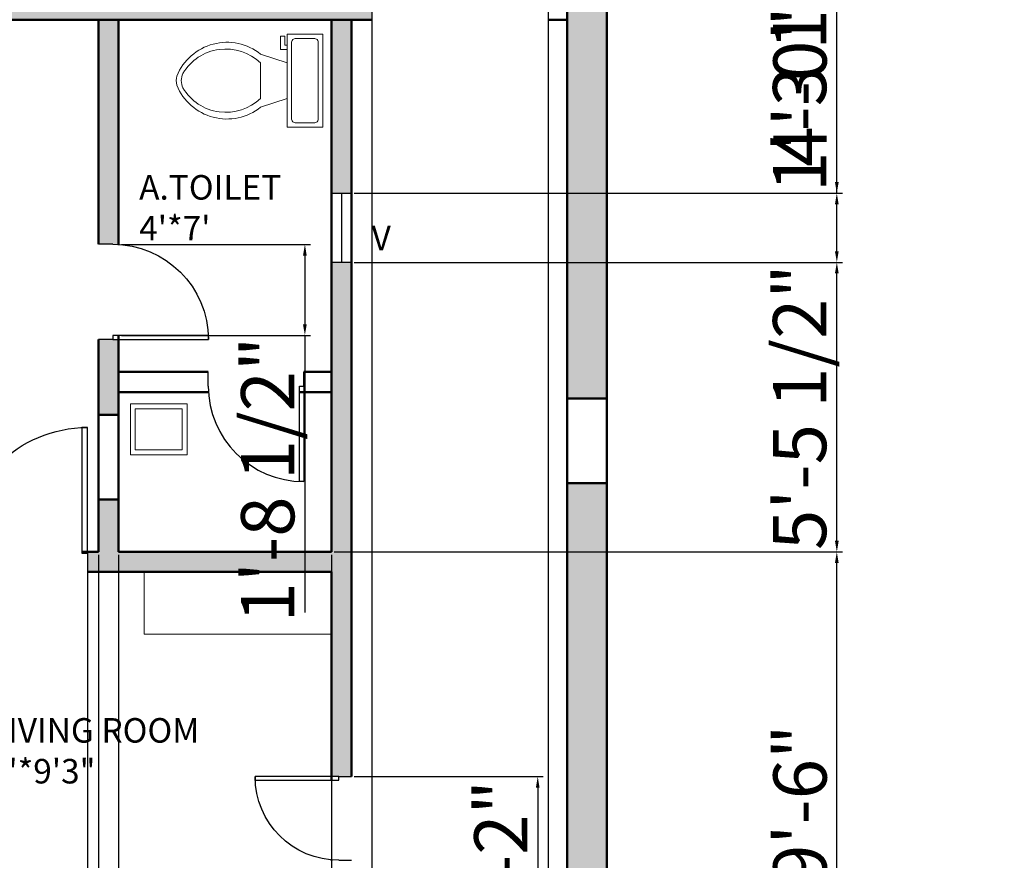
# Model space of a CAD drawing. Units: inches. Extents: x 2063 to 3370, y 2091 to 2971.
# Tile 5 of 14: x 2710 to 2932, y 2279 to 2468. Entities that reach past the tile are written whole.
import ezdxf

# ---------------------------------------------------------------- set-up
doc = ezdxf.new("R2010")
doc.units = ezdxf.units.IN
for name, color, linetype, lineweight in [('A-ANNO-DIMS', 2, 'Continuous', 18), ('A-ANNO-TEXT', 7, 'Continuous', 18), ('A-AREA-IDEN', 3, 'Continuous', 18), ('A-COLS', 7, 'Continuous', 50), ('A-DOOR', 4, 'Continuous', 25), ('A-FLOR-FIXT', 9, 'Continuous', 18), ('A-FURN', 8, 'Continuous', 18), ('A-GLAZ', 131, 'Continuous', 25), ('A-WALL', 7, 'Continuous', 50), ('A-WALL-PATT', 8, 'Continuous', 13)]:
    doc.layers.add(name, color=color, linetype=linetype, lineweight=lineweight)
doc.styles.get("Standard").update_dxf_attribs({"font": 'arial.ttf'})
doc.dimstyles.new('ISO-25', dxfattribs={"dimtxt": 12, "dimasz": 2.5, "dimexe": 1.25, "dimexo": 0.625, "dimtad": 1, "dimdec": 0, "dimlunit": 4, "dimtxsty": 'Standard', "dimcen": 2.5, "dimadec": 0, "dimazin": 0, "dimtfac": 1, "dimtdec": 0, "dimtmove": 0, "dimatfit": 3, "dimfxl": 1, "dimarcsym": 0})

# ---------------------------------------------------------------- blocks, each defined once
blk = doc.blocks.new('*U2')
for p, q in [((0, 0), (0, -6)), ((40, 0), (40, -6))]:
    blk.add_line(p, q)
blk.add_lwpolyline([(0, 0), (0, 40), (1.75, 40), (1.75, 0)], close=True)
blk.add_arc((0, 0), 40, 0, 90)
blk = doc.blocks.new('*U4')
for p, q in [((9.5, -6), (9.5, -2)), ((-10, -8.5), (-8, -8.5)), ((-10, -9.5), (-10, -8.5)), ((-8, -8.5), (-8, -8)), ((-7, -8), (-7, -9.5)), ((-4, -8), (-6, -14)), ((4, -8), (6, -14)), ((-7, -9.5), (-10, -9.5)), ((4, -14), (-4, -14))]:
    blk.add_line(p, q)
blk.add_lwpolyline([(10.5, -8), (10.5, 0), (-10.5, 0), (-10.5, -8)], close=True)
for points in [[(-9.5, -2), (-9.5, -6)], [(8.5, -1), (-8.5, -1)], [(-8.5, -7), (8.5, -7)]]:
    blk.add_lwpolyline(points)
for centre, radius, start, end in [((-8.62, -1.88), 0.884, 81.8699, 188.1301), ((8.62, -1.88), 0.884, 351.8699, 98.1301), ((-8.62, -6.12), 0.884, 171.8699, 278.1301), ((8.62, -6.12), 0.884, 261.8699, 8.1301), ((3.52, -21.58), 12.17, 141.4691, 247.9714), ((4.2, -21.82), 11.33, 136.3677, 238.9468), ((-3.52, -21.58), 12.17, 292.0284, 38.5307), ((-4.2, -21.82), 11.33, 301.053, 43.6321), ((0, -27.88), 4, 245.7318, 294.2682), ((0, -29), 4, 254.8605, 285.1395)]:
    blk.add_arc(centre, radius, start, end)
blk = doc.blocks.new('*D18')
at = {"layer": 'A-ANNO-DIMS', "color": 0, "lineweight": -2, "transparency": 16777216}
for p, q in [((2717.43, 2255.3), (2717.43, 2259.55)), ((2719.93, 2258.3), (2739.08, 2258.3)), ((2741.58, 2255.3), (2741.58, 2259.55)), ((2741.58, 2258.3), (2932.33, 2258.3))]:
    blk.add_line(p, q, dxfattribs=at)
at = {"layer": 'A-ANNO-DIMS', "color": 0, "transparency": 16777216}
for points in [[(2719.93, 2258.72), (2719.93, 2257.88), (2717.43, 2258.3)], [(2739.08, 2258.72), (2739.08, 2257.88), (2741.58, 2258.3)]]:
    blk.add_solid(points, dxfattribs=at)
at = {"layer": 'Defpoints', "color": 0, "transparency": 16777216}
for p in [(2741.58, 2258.3), (2717.43, 2254.68), (2741.58, 2254.68)]:
    blk.add_point(p, dxfattribs=at)
at = {"layer": 'A-ANNO-DIMS', "color": 0, "transparency": 16777216, "insert": (2838.21, 2265.13), "char_height": 12, "attachment_point": 5}
blk.add_mtext('2-SEAT SOFA 2\'-0" TYP.', dxfattribs=at)
blk = doc.blocks.new('*D28')
at = {"layer": 'A-ANNO-DIMS', "color": 0, "lineweight": -2, "transparency": 16777216}
for p, q in [((2647.53, 2480.55), (2647.53, 2476.06)), ((2673.28, 2480.55), (2673.28, 2476.06)), ((2650.03, 2477.31), (2670.78, 2477.31)), ((2673.28, 2477.31), (2793.91, 2477.31))]:
    blk.add_line(p, q, dxfattribs=at)
at = {"layer": 'A-ANNO-DIMS', "color": 0, "transparency": 16777216}
for points in [[(2650.03, 2477.73), (2650.03, 2476.9), (2647.53, 2477.31)], [(2670.78, 2477.73), (2670.78, 2476.9), (2673.28, 2477.31)]]:
    blk.add_solid(points, dxfattribs=at)
at = {"layer": 'Defpoints', "color": 0, "transparency": 16777216}
for p in [(2647.53, 2481.18), (2673.28, 2481.18), (2673.28, 2477.31)]:
    blk.add_point(p, dxfattribs=at)
at = {"layer": 'A-ANNO-DIMS', "color": 0, "transparency": 16777216, "insert": (2734.85, 2484.14), "char_height": 12, "attachment_point": 5}
blk.add_mtext('SINK 2\'-2" TYP.', dxfattribs=at)
blk = doc.blocks.new('*D94')
at = {"layer": 'A-ANNO-DIMS', "color": 0, "lineweight": -2, "transparency": 16777216}
for p, q in [((2611.75, 2347.8), (2611.75, 2101.18)), ((2728.14, 2347.8), (2728.14, 2101.18)), ((2614.25, 2102.43), (2725.64, 2102.43))]:
    blk.add_line(p, q, dxfattribs=at)
at = {"layer": 'A-ANNO-DIMS', "color": 0, "transparency": 16777216}
for points in [[(2614.25, 2102.84), (2614.25, 2102.01), (2611.75, 2102.43)], [(2725.64, 2102.84), (2725.64, 2102.01), (2728.14, 2102.43)]]:
    blk.add_solid(points, dxfattribs=at)
at = {"layer": 'Defpoints', "color": 0, "transparency": 16777216}
for p in [(2611.75, 2348.43), (2728.14, 2348.43), (2728.14, 2102.43)]:
    blk.add_point(p, dxfattribs=at)
at = {"layer": 'A-ANNO-DIMS', "color": 0, "transparency": 16777216, "insert": (2669.94, 2109.26), "char_height": 12, "attachment_point": 5}
blk.add_mtext('9\'-8 1/2"', dxfattribs=at)
blk = doc.blocks.new('*D95')
at = {"layer": 'A-ANNO-DIMS', "color": 0, "lineweight": -2, "transparency": 16777216}
for p, q in [((2728.14, 2347.8), (2728.14, 2101.18)), ((2732.64, 2347.8), (2732.64, 2101.18)), ((2725.64, 2102.43), (2723.14, 2102.43)), ((2728.14, 2102.43), (2732.64, 2102.43)), ((2735.14, 2102.43), (2798.75, 2102.43))]:
    blk.add_line(p, q, dxfattribs=at)
at = {"layer": 'A-ANNO-DIMS', "color": 0, "transparency": 16777216}
for points in [[(2725.64, 2102.84), (2725.64, 2102.01), (2728.14, 2102.43)], [(2735.14, 2102.84), (2735.14, 2102.01), (2732.64, 2102.43)]]:
    blk.add_solid(points, dxfattribs=at)
at = {"layer": 'Defpoints', "color": 0, "transparency": 16777216}
for p in [(2728.14, 2348.43), (2732.64, 2348.43), (2732.64, 2102.43)]:
    blk.add_point(p, dxfattribs=at)
at = {"layer": 'A-ANNO-DIMS', "color": 0, "transparency": 16777216, "insert": (2768.19, 2109.26), "char_height": 12, "attachment_point": 5}
blk.add_mtext('0\'-4 1/2"', dxfattribs=at)
blk = doc.blocks.new('*D96')
at = {"layer": 'A-ANNO-DIMS', "color": 0, "lineweight": -2, "transparency": 16777216}
for p, q in [((2732.64, 2347.8), (2732.64, 2101.18)), ((2780.64, 2347.8), (2780.64, 2101.18)), ((2735.14, 2102.43), (2778.14, 2102.43))]:
    blk.add_line(p, q, dxfattribs=at)
at = {"layer": 'A-ANNO-DIMS', "color": 0, "transparency": 16777216}
for points in [[(2735.14, 2102.84), (2735.14, 2102.01), (2732.64, 2102.43)], [(2778.14, 2102.84), (2778.14, 2102.01), (2780.64, 2102.43)]]:
    blk.add_solid(points, dxfattribs=at)
at = {"layer": 'Defpoints', "color": 0, "transparency": 16777216}
for p in [(2732.64, 2348.43), (2780.64, 2348.43), (2780.64, 2102.43)]:
    blk.add_point(p, dxfattribs=at)
at = {"layer": 'A-ANNO-DIMS', "color": 0, "transparency": 16777216, "insert": (2756.64, 2109.18), "char_height": 12, "attachment_point": 5}
blk.add_mtext('4\'-0"', dxfattribs=at)
blk = doc.blocks.new('*D113')
at = {"layer": 'A-ANNO-DIMS', "color": 0, "lineweight": -2, "transparency": 16777216}
for p, q in [((2781.26, 2348.43), (2895.82, 2348.43)), ((2894.57, 2236.93), (2894.57, 2345.93)), ((2781.26, 2234.43), (2895.82, 2234.43))]:
    blk.add_line(p, q, dxfattribs=at)
at = {"layer": 'A-ANNO-DIMS', "color": 0, "transparency": 16777216}
for points in [[(2894.15, 2345.93), (2894.99, 2345.93), (2894.57, 2348.43)], [(2894.15, 2236.93), (2894.99, 2236.93), (2894.57, 2234.43)]]:
    blk.add_solid(points, dxfattribs=at)
at = {"layer": 'Defpoints', "color": 0, "transparency": 16777216}
for p in [(2780.64, 2348.43), (2894.57, 2348.43), (2780.64, 2234.43)]:
    blk.add_point(p, dxfattribs=at)
at = {"layer": 'A-ANNO-DIMS', "color": 0, "transparency": 16777216, "insert": (2887.82, 2291.43), "char_height": 12, "attachment_point": 5, "rotation": 90}
blk.add_mtext('9\'-6"', dxfattribs=at)
blk = doc.blocks.new('*D114')
at = {"layer": 'A-ANNO-DIMS', "color": 0, "lineweight": -2, "transparency": 16777216}
for p, q in [((2785.76, 2413.72), (2895.82, 2413.72)), ((2894.57, 2350.93), (2894.57, 2411.22)), ((2781.26, 2348.43), (2895.82, 2348.43))]:
    blk.add_line(p, q, dxfattribs=at)
at = {"layer": 'A-ANNO-DIMS', "color": 0, "transparency": 16777216}
for points in [[(2894.15, 2411.22), (2894.99, 2411.22), (2894.57, 2413.72)], [(2894.15, 2350.93), (2894.99, 2350.93), (2894.57, 2348.43)]]:
    blk.add_solid(points, dxfattribs=at)
at = {"layer": 'Defpoints', "color": 0, "transparency": 16777216}
for p in [(2785.14, 2413.72), (2894.57, 2413.72), (2780.64, 2348.43)]:
    blk.add_point(p, dxfattribs=at)
at = {"layer": 'A-ANNO-DIMS', "color": 0, "transparency": 16777216, "insert": (2887.74, 2381.07), "char_height": 12, "attachment_point": 5, "rotation": 90}
blk.add_mtext('5\'-5 1/2"', dxfattribs=at)
blk = doc.blocks.new('*D115')
at = {"layer": 'A-ANNO-DIMS', "color": 0, "lineweight": -2, "transparency": 16777216}
for p, q in [((2894.57, 2429.31), (2894.57, 2491.79)), ((2785.76, 2429.31), (2895.82, 2429.31)), ((2894.57, 2416.22), (2894.57, 2426.81)), ((2785.76, 2413.72), (2895.82, 2413.72))]:
    blk.add_line(p, q, dxfattribs=at)
at = {"layer": 'A-ANNO-DIMS', "color": 0, "transparency": 16777216}
for points in [[(2894.15, 2426.81), (2894.99, 2426.81), (2894.57, 2429.31)], [(2894.15, 2416.22), (2894.99, 2416.22), (2894.57, 2413.72)]]:
    blk.add_solid(points, dxfattribs=at)
at = {"layer": 'Defpoints', "color": 0, "transparency": 16777216}
for p in [(2785.14, 2429.31), (2894.57, 2429.31), (2785.14, 2413.72)]:
    blk.add_point(p, dxfattribs=at)
at = {"layer": 'A-ANNO-DIMS', "color": 0, "transparency": 16777216, "insert": (2887.74, 2461.8), "char_height": 12, "attachment_point": 5, "rotation": 90}
blk.add_mtext('1\'-3 1/2"', dxfattribs=at)
blk = doc.blocks.new('*D116')
at = {"layer": 'A-ANNO-DIMS', "color": 0, "lineweight": -2, "transparency": 16777216}
for p, q in [((2790.36, 2477.43), (2895.82, 2477.43)), ((2894.57, 2431.81), (2894.57, 2474.93)), ((2785.76, 2429.31), (2895.82, 2429.31))]:
    blk.add_line(p, q, dxfattribs=at)
at = {"layer": 'A-ANNO-DIMS', "color": 0, "transparency": 16777216}
for points in [[(2894.15, 2474.93), (2894.99, 2474.93), (2894.57, 2477.43)], [(2894.15, 2431.81), (2894.99, 2431.81), (2894.57, 2429.31)]]:
    blk.add_solid(points, dxfattribs=at)
at = {"layer": 'Defpoints', "color": 0, "transparency": 16777216}
for p in [(2789.73, 2477.43), (2894.57, 2477.43), (2785.14, 2429.31)]:
    blk.add_point(p, dxfattribs=at)
at = {"layer": 'A-ANNO-DIMS', "color": 0, "transparency": 16777216, "insert": (2887.82, 2453.37), "char_height": 12, "attachment_point": 5, "rotation": 90}
blk.add_mtext('4\'-0"', dxfattribs=at)
blk = doc.blocks.new('*D131')
at = {"layer": 'A-ANNO-DIMS', "color": 0, "lineweight": -2, "transparency": 16777216}
for p, q in [((2789.73, 2476.8), (2789.73, 2101.18)), ((2829.49, 2470.78), (2829.49, 2101.18)), ((2792.23, 2102.43), (2826.99, 2102.43))]:
    blk.add_line(p, q, dxfattribs=at)
at = {"layer": 'A-ANNO-DIMS', "color": 0, "transparency": 16777216}
for points in [[(2792.23, 2102.84), (2792.23, 2102.01), (2789.73, 2102.43)], [(2826.99, 2102.84), (2826.99, 2102.01), (2829.49, 2102.43)]]:
    blk.add_solid(points, dxfattribs=at)
at = {"layer": 'Defpoints', "color": 0, "transparency": 16777216}
for p in [(2789.73, 2477.43), (2829.49, 2471.41), (2829.49, 2102.43)]:
    blk.add_point(p, dxfattribs=at)
at = {"layer": 'A-ANNO-DIMS', "color": 0, "transparency": 16777216, "insert": (2809.61, 2109.18), "char_height": 12, "attachment_point": 5}
blk.add_mtext('3\'-4"', dxfattribs=at)
blk = doc.blocks.new('*D132')
at = {"layer": 'A-ANNO-DIMS', "color": 0, "lineweight": -2, "transparency": 16777216}
for p, q in [((2697.29, 2347.55), (2697.29, 2101.18)), ((2725.61, 2347.55), (2725.61, 2101.18)), ((2699.79, 2102.43), (2723.11, 2102.43)), ((2725.61, 2102.43), (2789.42, 2102.43))]:
    blk.add_line(p, q, dxfattribs=at)
at = {"layer": 'A-ANNO-DIMS', "color": 0, "transparency": 16777216}
for points in [[(2699.79, 2102.84), (2699.79, 2102.01), (2697.29, 2102.43)], [(2723.11, 2102.84), (2723.11, 2102.01), (2725.61, 2102.43)]]:
    blk.add_solid(points, dxfattribs=at)
at = {"layer": 'Defpoints', "color": 0, "transparency": 16777216}
for p in [(2697.29, 2348.17), (2725.61, 2348.17), (2725.61, 2102.43)]:
    blk.add_point(p, dxfattribs=at)
at = {"layer": 'A-ANNO-DIMS', "color": 0, "transparency": 16777216, "insert": (2758.77, 2109.26), "char_height": 12, "attachment_point": 5}
blk.add_mtext('2\'-4 1/2"', dxfattribs=at)
blk = doc.blocks.new('*D133')
at = {"layer": 'A-ANNO-DIMS', "color": 0, "lineweight": -2, "transparency": 16777216}
for p, q in [((2733.26, 2417.76), (2775.89, 2417.76)), ((2774.64, 2415.26), (2774.64, 2399.73)), ((2733.26, 2397.23), (2775.89, 2397.23)), ((2774.64, 2397.23), (2774.64, 2334.75))]:
    blk.add_line(p, q, dxfattribs=at)
at = {"layer": 'A-ANNO-DIMS', "color": 0, "transparency": 16777216}
for points in [[(2774.22, 2415.26), (2775.05, 2415.26), (2774.64, 2417.76)], [(2774.22, 2399.73), (2775.05, 2399.73), (2774.64, 2397.23)]]:
    blk.add_solid(points, dxfattribs=at)
at = {"layer": 'Defpoints', "color": 0, "transparency": 16777216}
for p in [(2732.64, 2417.76), (2732.64, 2397.23), (2774.64, 2397.23)]:
    blk.add_point(p, dxfattribs=at)
at = {"layer": 'A-ANNO-DIMS', "color": 0, "transparency": 16777216, "insert": (2767.81, 2364.74), "char_height": 12, "attachment_point": 5, "rotation": 90}
blk.add_mtext('1\'-8 1/2"', dxfattribs=at)
blk = doc.blocks.new('*D134')
at = {"layer": 'A-ANNO-DIMS', "color": 0, "lineweight": -2, "transparency": 16777216}
for p, q in [((2785.76, 2297.78), (2828.39, 2297.78)), ((2827.14, 2295.28), (2827.14, 2262.52)), ((2785.76, 2260.02), (2828.39, 2260.02))]:
    blk.add_line(p, q, dxfattribs=at)
at = {"layer": 'A-ANNO-DIMS', "color": 0, "transparency": 16777216}
for points in [[(2826.72, 2295.28), (2827.55, 2295.28), (2827.14, 2297.78)], [(2826.72, 2262.52), (2827.55, 2262.52), (2827.14, 2260.02)]]:
    blk.add_solid(points, dxfattribs=at)
at = {"layer": 'Defpoints', "color": 0, "transparency": 16777216}
for p in [(2785.14, 2297.78), (2785.14, 2260.02), (2827.14, 2260.02)]:
    blk.add_point(p, dxfattribs=at)
at = {"layer": 'A-ANNO-DIMS', "color": 0, "transparency": 16777216, "insert": (2820.38, 2278.9), "char_height": 12, "attachment_point": 5, "rotation": 90}
blk.add_mtext('3\'-2"', dxfattribs=at)

msp = doc.modelspace()

# ---------------------------------------------------------------- hatches: boundary and pattern name
at = {"layer": 'A-WALL-PATT'}
h = msp.add_hatch(color=256, dxfattribs=at)
h.dxf.hatch_style = 1
h.paths.add_polyline_path([(2842.75, 2864.43), (2602.75, 2864.43), (2602.75, 2831.43), (2608.62, 2831.43), (2608.62, 2859.54), (2836.36, 2859.54), (2836.36, 2831.15), (2842.75, 2831.15)])
h.paths.add_polyline_path([(2775.49, 2177.04), (2815.13, 2177.04), (2815.13, 2197.65), (2775.49, 2197.65)], flags=9)
h.paths.add_polyline_path([(2634.18, 2285.75), (2670.81, 2285.75), (2670.81, 2306.35), (2634.18, 2306.35)], flags=9)
h.paths.add_polyline_path([(2701.65, 2293.1), (2755.85, 2293.1), (2755.85, 2313.71), (2701.65, 2313.71)], flags=9)
h.paths.add_polyline_path([(2735.8, 2415.55), (2772.95, 2415.55), (2772.95, 2436.13), (2735.8, 2436.13)], flags=9)
h.paths.add_polyline_path([(2641.75, 2422.21), (2718.67, 2422.21), (2718.67, 2442.82), (2641.75, 2442.82)], flags=9)
h.paths.add_polyline_path([(2710.43, 2552.92), (2764.91, 2552.92), (2764.91, 2573.53), (2710.43, 2573.53)], flags=9)
h.paths.add_polyline_path([(2625.23, 2527.83), (2661.86, 2527.83), (2661.86, 2548.44), (2625.23, 2548.44)], flags=9)
h.paths.add_polyline_path([(2627.53, 2598.16), (2652.13, 2598.16), (2652.13, 2618.77), (2627.53, 2618.77)], flags=9)
h.paths.add_polyline_path([(2646.64, 2696.08), (2723.56, 2696.08), (2723.56, 2716.69), (2646.64, 2716.69)], flags=9)
h.paths.add_polyline_path([(2791.65, 2795.64), (2828.72, 2795.64), (2828.72, 2807.02), (2791.65, 2807.02)], flags=9)
h.paths.add_polyline_path([(2751.88, 2214.78), (2761.93, 2214.78), (2761.93, 2226.17), (2751.88, 2226.17)], flags=9)
h.paths.add_polyline_path([(2664.96, 2215.71), (2675, 2215.71), (2675, 2227.09), (2664.96, 2227.09)], flags=9)
h.paths.add_polyline_path([(2788.26, 2413.43), (2796.17, 2413.43), (2796.17, 2424.82), (2788.26, 2424.82)], flags=9)
h.paths.add_polyline_path([(2728.86, 2795.64), (2765.93, 2795.64), (2765.93, 2807.02), (2728.86, 2807.02)], flags=9)
h.paths.add_polyline_path([(2760.39, 2726.09), (2823.16, 2726.09), (2823.16, 2746.7), (2760.39, 2746.7)], flags=9)
h = msp.add_hatch(color=256, dxfattribs=at)
h.dxf.hatch_style = 1
h.paths.add_polyline_path([(2290.22, 2192.43), (2278.22, 2192.43), (2182.22, 2192.43), (2182.22, 2189.43), (2182.22, 2187.43), (2278.22, 2187.43), (2290.22, 2187.42)])
h.paths.add_polyline_path([(2748.25, 2192.43), (2736.25, 2192.43), (2640.25, 2192.43), (2640.25, 2189.43), (2640.25, 2187.43), (2736.25, 2187.43), (2748.25, 2187.42)], flags=17)
h.paths.add_polyline_path([(2653.66, 2234.43), (2611.75, 2234.43), (2611.75, 2232.93), (2611.75, 2225.43), (2653.66, 2225.43)])
h.paths.add_polyline_path([(2717.13, 2234.43), (2675.81, 2234.43), (2675.81, 2225.43), (2717.13, 2225.43)])
h.paths.add_polyline_path([(2611.75, 2222.57), (2602.75, 2222.57), (2602.75, 2144.43), (2842.75, 2144.43), (2842.75, 2220.3), (2833.75, 2220.3), (2833.75, 2153.43), (2829.39, 2153.43), (2754.78, 2153.43), (2611.75, 2153.43)])
h.paths.add_polyline_path([(2687.64, 2308.91), (2683.14, 2308.91), (2683.14, 2234.43), (2687.64, 2234.43)])
h.paths.add_polyline_path([(2744.5, 2234.43), (2736.25, 2234.43), (2736.25, 2225.43), (2744.5, 2225.43)])
h.paths.add_polyline_path([(2785.14, 2260.02), (2782.31, 2260.02), (2780.64, 2260.02), (2780.64, 2234.43), (2766.65, 2234.43), (2766.65, 2225.43), (2785.14, 2225.43)])
h.paths.add_polyline_path([(2842.75, 2363.93), (2833.75, 2363.93), (2833.75, 2239.41), (2842.75, 2239.41)])
h.paths.add_polyline_path([(2775.49, 2177.04), (2815.13, 2177.04), (2815.13, 2197.65), (2775.49, 2197.65)], flags=25)
h.paths.add_polyline_path([(2634.18, 2285.75), (2670.81, 2285.75), (2670.81, 2306.35), (2634.18, 2306.35)], flags=9)
h.paths.add_polyline_path([(2701.65, 2293.1), (2755.85, 2293.1), (2755.85, 2313.71), (2701.65, 2313.71)], flags=9)
h.paths.add_polyline_path([(2735.8, 2415.55), (2772.95, 2415.55), (2772.95, 2436.13), (2735.8, 2436.13)], flags=9)
h.paths.add_polyline_path([(2641.75, 2422.21), (2718.67, 2422.21), (2718.67, 2442.82), (2641.75, 2442.82)], flags=9)
h.paths.add_polyline_path([(2710.43, 2552.92), (2764.91, 2552.92), (2764.91, 2573.53), (2710.43, 2573.53)], flags=9)
h.paths.add_polyline_path([(2625.23, 2527.83), (2661.86, 2527.83), (2661.86, 2548.44), (2625.23, 2548.44)], flags=9)
h.paths.add_polyline_path([(2627.53, 2598.16), (2652.13, 2598.16), (2652.13, 2618.77), (2627.53, 2618.77)], flags=9)
h.paths.add_polyline_path([(2646.64, 2696.08), (2723.56, 2696.08), (2723.56, 2716.69), (2646.64, 2716.69)], flags=9)
h.paths.add_polyline_path([(2791.65, 2795.64), (2828.72, 2795.64), (2828.72, 2807.02), (2791.65, 2807.02)], flags=9)
h.paths.add_polyline_path([(2751.88, 2214.78), (2761.93, 2214.78), (2761.93, 2226.17), (2751.88, 2226.17)], flags=9)
h.paths.add_polyline_path([(2788.26, 2413.43), (2796.17, 2413.43), (2796.17, 2424.82), (2788.26, 2424.82)], flags=9)
h.paths.add_polyline_path([(2761.97, 2835.24), (2769.88, 2835.24), (2769.88, 2846.62), (2761.97, 2846.62)], flags=9)
h.paths.add_polyline_path([(2675.89, 2833.68), (2685.93, 2833.68), (2685.93, 2845.06), (2675.89, 2845.06)], flags=9)
h.paths.add_polyline_path([(2728.86, 2795.64), (2765.93, 2795.64), (2765.93, 2807.02), (2728.86, 2807.02)], flags=9)
h.paths.add_polyline_path([(2760.39, 2726.09), (2823.16, 2726.09), (2823.16, 2746.7), (2760.39, 2746.7)], flags=9)
h = msp.add_hatch(color=256, dxfattribs=at)
h.dxf.hatch_style = 1
h.paths.add_polyline_path([(2680.75, 2631.93), (2684.44, 2631.93), (2684.44, 2636.43), (2683.1, 2636.43), (2611.75, 2636.43), (2611.75, 2631.93), (2648.72, 2631.93), (2671.75, 2631.93), (2676.25, 2631.93), (2676.25, 2623.58), (2678.23, 2623.58), (2680.75, 2623.58)])
h.paths.add_polyline_path([(2728.75, 2636.43), (2724.44, 2636.43), (2724.44, 2631.93), (2728.75, 2631.93)])
h.paths.add_polyline_path([(2772.02, 2636.43), (2733.25, 2636.43), (2733.25, 2631.93), (2772.02, 2631.93)])
h.paths.add_polyline_path([(2733.25, 2636.43), (2728.75, 2636.43), (2728.75, 2631.93), (2733.25, 2631.93)])
h.paths.add_polyline_path([(2833.75, 2636.43), (2812.02, 2636.43), (2812.02, 2631.93), (2833.75, 2631.93)])
h.paths.add_polyline_path([(2842.75, 2626.16), (2833.75, 2626.16), (2833.75, 2585.28), (2842.75, 2585.28)])
h.paths.add_polyline_path([(2842.75, 2679.03), (2833.75, 2679.03), (2833.75, 2645.28), (2842.75, 2645.28)])
h.paths.add_polyline_path([(2611.75, 2619.52), (2602.75, 2619.52), (2602.75, 2548.5), (2611.75, 2548.5), (2611.75, 2579.43)])
h.paths.add_polyline_path([(2646.64, 2696.08), (2723.56, 2696.08), (2723.56, 2716.69), (2646.64, 2716.69)], flags=9)
h.paths.add_polyline_path([(2791.65, 2795.64), (2828.72, 2795.64), (2828.72, 2807.02), (2791.65, 2807.02)], flags=9)
h.paths.add_polyline_path([(2761.97, 2835.24), (2769.88, 2835.24), (2769.88, 2846.62), (2761.97, 2846.62)], flags=9)
h.paths.add_polyline_path([(2675.89, 2833.68), (2685.93, 2833.68), (2685.93, 2845.06), (2675.89, 2845.06)], flags=9)
h.paths.add_polyline_path([(2728.86, 2795.64), (2765.93, 2795.64), (2765.93, 2807.02), (2728.86, 2807.02)], flags=9)
h.paths.add_polyline_path([(2775.49, 2177.04), (2815.13, 2177.04), (2815.13, 2197.65), (2775.49, 2197.65)], flags=9)
h.paths.add_polyline_path([(2634.18, 2285.75), (2670.81, 2285.75), (2670.81, 2306.35), (2634.18, 2306.35)], flags=9)
h.paths.add_polyline_path([(2701.65, 2293.1), (2755.85, 2293.1), (2755.85, 2313.71), (2701.65, 2313.71)], flags=9)
h.paths.add_polyline_path([(2735.8, 2415.55), (2772.95, 2415.55), (2772.95, 2436.13), (2735.8, 2436.13)], flags=9)
h.paths.add_polyline_path([(2641.75, 2422.21), (2718.67, 2422.21), (2718.67, 2442.82), (2641.75, 2442.82)], flags=9)
h.paths.add_polyline_path([(2710.43, 2552.92), (2764.91, 2552.92), (2764.91, 2573.53), (2710.43, 2573.53)], flags=9)
h.paths.add_polyline_path([(2625.23, 2527.83), (2661.86, 2527.83), (2661.86, 2548.44), (2625.23, 2548.44)], flags=9)
h.paths.add_polyline_path([(2751.88, 2214.78), (2761.93, 2214.78), (2761.93, 2226.17), (2751.88, 2226.17)], flags=9)
h.paths.add_polyline_path([(2664.96, 2215.71), (2675, 2215.71), (2675, 2227.09), (2664.96, 2227.09)], flags=9)
h.paths.add_polyline_path([(2788.26, 2413.43), (2796.17, 2413.43), (2796.17, 2424.82), (2788.26, 2424.82)], flags=9)
h = msp.add_hatch(color=256, dxfattribs=at)
h.dxf.hatch_style = 1
h.paths.add_polyline_path([(2611.75, 2343.93), (2611.75, 2477.43), (2611.75, 2514.15), (2602.75, 2514.15), (2602.75, 2241.68), (2611.75, 2241.68), (2611.75, 2258.43)])
h.paths.add_polyline_path([(2775.49, 2177.04), (2815.13, 2177.04), (2815.13, 2197.65), (2775.49, 2197.65)], flags=9)
h.paths.add_polyline_path([(2735.8, 2415.55), (2772.95, 2415.55), (2772.95, 2436.13), (2735.8, 2436.13)], flags=9)
h.paths.add_polyline_path([(2641.75, 2422.21), (2718.67, 2422.21), (2718.67, 2442.82), (2641.75, 2442.82)], flags=9)
h.paths.add_polyline_path([(2710.43, 2552.92), (2764.91, 2552.92), (2764.91, 2573.53), (2710.43, 2573.53)], flags=9)
h.paths.add_polyline_path([(2625.23, 2527.83), (2661.86, 2527.83), (2661.86, 2548.44), (2625.23, 2548.44)], flags=9)
h.paths.add_polyline_path([(2627.53, 2598.16), (2652.13, 2598.16), (2652.13, 2618.77), (2627.53, 2618.77)], flags=9)
h.paths.add_polyline_path([(2646.64, 2696.08), (2723.56, 2696.08), (2723.56, 2716.69), (2646.64, 2716.69)], flags=9)
h.paths.add_polyline_path([(2791.65, 2795.64), (2828.72, 2795.64), (2828.72, 2807.02), (2791.65, 2807.02)], flags=9)
h.paths.add_polyline_path([(2751.88, 2214.78), (2761.93, 2214.78), (2761.93, 2226.17), (2751.88, 2226.17)], flags=9)
h.paths.add_polyline_path([(2788.26, 2413.43), (2796.17, 2413.43), (2796.17, 2424.82), (2788.26, 2424.82)], flags=9)
h.paths.add_polyline_path([(2761.97, 2835.24), (2769.88, 2835.24), (2769.88, 2846.62), (2761.97, 2846.62)], flags=9)
h.paths.add_polyline_path([(2675.89, 2833.68), (2685.93, 2833.68), (2685.93, 2845.06), (2675.89, 2845.06)], flags=9)
h.paths.add_polyline_path([(2728.86, 2795.64), (2765.93, 2795.64), (2765.93, 2807.02), (2728.86, 2807.02)], flags=9)
h.paths.add_polyline_path([(2760.39, 2726.09), (2823.16, 2726.09), (2823.16, 2746.7), (2760.39, 2746.7)], flags=9)
h = msp.add_hatch(color=256, dxfattribs=at)
h.dxf.hatch_style = 1
h.paths.add_polyline_path([(2785.14, 2468.43), (2780.64, 2468.43), (2780.64, 2429.31), (2785.14, 2429.31)])
h.paths.add_polyline_path([(2842.75, 2525.28), (2833.75, 2525.28), (2833.75, 2523.93), (2833.75, 2466.93), (2833.75, 2383.04), (2842.75, 2383.04)])
h.paths.add_polyline_path([(2789.73, 2477.43), (2680.75, 2477.43), (2680.75, 2579.43), (2680.75, 2589.96), (2678.23, 2589.96), (2676.25, 2589.96), (2676.25, 2583.93), (2667.25, 2583.93), (2611.75, 2583.93), (2611.75, 2579.43), (2671.75, 2579.43), (2676.25, 2579.43), (2676.25, 2477.43), (2611.75, 2477.43), (2611.75, 2468.43), (2728.75, 2468.43), (2789.73, 2468.43), (2789.73, 2471.41)])
h.paths.add_polyline_path([(2710.43, 2552.92), (2764.91, 2552.92), (2764.91, 2573.53), (2710.43, 2573.53)], flags=25)
h.paths.add_polyline_path([(2625.23, 2527.83), (2661.86, 2527.83), (2661.86, 2548.44), (2625.23, 2548.44)], flags=25)
h.paths.add_polyline_path([(2627.53, 2598.16), (2652.13, 2598.16), (2652.13, 2618.77), (2627.53, 2618.77)], flags=9)
h.paths.add_polyline_path([(2646.64, 2696.08), (2723.56, 2696.08), (2723.56, 2716.69), (2646.64, 2716.69)], flags=9)
h.paths.add_polyline_path([(2791.65, 2795.64), (2828.72, 2795.64), (2828.72, 2807.02), (2791.65, 2807.02)], flags=9)
h.paths.add_polyline_path([(2761.97, 2835.24), (2769.88, 2835.24), (2769.88, 2846.62), (2761.97, 2846.62)], flags=9)
h.paths.add_polyline_path([(2675.89, 2833.68), (2685.93, 2833.68), (2685.93, 2845.06), (2675.89, 2845.06)], flags=9)
h.paths.add_polyline_path([(2728.86, 2795.64), (2765.93, 2795.64), (2765.93, 2807.02), (2728.86, 2807.02)], flags=9)
h.paths.add_polyline_path([(2760.39, 2726.09), (2823.16, 2726.09), (2823.16, 2746.7), (2760.39, 2746.7)], flags=9)
h.paths.add_polyline_path([(2775.49, 2177.04), (2815.13, 2177.04), (2815.13, 2197.65), (2775.49, 2197.65)], flags=9)
h.paths.add_polyline_path([(2634.18, 2285.75), (2670.81, 2285.75), (2670.81, 2306.35), (2634.18, 2306.35)], flags=9)
h.paths.add_polyline_path([(2701.65, 2293.1), (2755.85, 2293.1), (2755.85, 2313.71), (2701.65, 2313.71)], flags=9)
h.paths.add_polyline_path([(2641.75, 2422.21), (2718.67, 2422.21), (2718.67, 2442.82), (2641.75, 2442.82)], flags=9)
h.paths.add_polyline_path([(2751.88, 2214.78), (2761.93, 2214.78), (2761.93, 2226.17), (2751.88, 2226.17)], flags=9)
h.paths.add_polyline_path([(2664.96, 2215.71), (2675, 2215.71), (2675, 2227.09), (2664.96, 2227.09)], flags=9)
h.paths.add_polyline_path([(2788.26, 2413.43), (2796.17, 2413.43), (2796.17, 2424.82), (2788.26, 2424.82)], flags=9)
h = msp.add_hatch(color=256, dxfattribs=at)
h.dxf.hatch_style = 1
h.paths.add_polyline_path([(2785.14, 2343.93), (2785.14, 2392.49), (2785.14, 2413.72), (2780.64, 2413.72), (2780.64, 2384.43), (2780.64, 2348.43), (2732.64, 2348.43), (2732.64, 2360.22), (2728.14, 2360.22), (2728.14, 2348.43), (2725.61, 2348.43), (2725.61, 2348.17), (2725.61, 2343.93), (2780.64, 2343.93), (2780.64, 2329.91), (2780.64, 2297.78), (2782.31, 2297.78), (2785.14, 2297.78)])
h.paths.add_polyline_path([(2732.64, 2396.29), (2731.36, 2396.29), (2728.14, 2396.29), (2728.14, 2379.34), (2732.64, 2379.34)], flags=17)
h.paths.add_polyline_path([(2732.64, 2468.43), (2728.14, 2468.43), (2728.14, 2417.8), (2731.36, 2417.8, -0.014809), (2732.64, 2417.76)])
h.paths.add_polyline_path([(2697.29, 2348.43), (2611.75, 2348.43), (2611.75, 2343.93), (2683.14, 2343.93), (2697.29, 2343.93)])
h.paths.add_polyline_path([(2710.43, 2552.92), (2764.91, 2552.92), (2764.91, 2573.53), (2710.43, 2573.53)], flags=9)
h.paths.add_polyline_path([(2625.23, 2527.83), (2661.86, 2527.83), (2661.86, 2548.44), (2625.23, 2548.44)], flags=9)
h.paths.add_polyline_path([(2627.53, 2598.16), (2652.13, 2598.16), (2652.13, 2618.77), (2627.53, 2618.77)], flags=9)
h.paths.add_polyline_path([(2646.64, 2696.08), (2723.56, 2696.08), (2723.56, 2716.69), (2646.64, 2716.69)], flags=9)
h.paths.add_polyline_path([(2791.65, 2795.64), (2828.72, 2795.64), (2828.72, 2807.02), (2791.65, 2807.02)], flags=9)
h.paths.add_polyline_path([(2761.97, 2835.24), (2769.88, 2835.24), (2769.88, 2846.62), (2761.97, 2846.62)], flags=9)
h.paths.add_polyline_path([(2675.89, 2833.68), (2685.93, 2833.68), (2685.93, 2845.06), (2675.89, 2845.06)], flags=9)
h.paths.add_polyline_path([(2728.86, 2795.64), (2765.93, 2795.64), (2765.93, 2807.02), (2728.86, 2807.02)], flags=9)
h.paths.add_polyline_path([(2760.39, 2726.09), (2823.16, 2726.09), (2823.16, 2746.7), (2760.39, 2746.7)], flags=9)
h = msp.add_hatch(color=256, dxfattribs=at)
h.dxf.hatch_style = 1
h.paths.add_polyline_path([(2655.27, 2831.43), (2611.75, 2831.43), (2611.75, 2822.43), (2655.27, 2822.43)])
h.paths.add_polyline_path([(2722.06, 2831.43), (2703.27, 2831.43), (2703.27, 2822.43), (2722.06, 2822.43)])
h.paths.add_polyline_path([(2754.66, 2831.43), (2741.18, 2831.43), (2741.18, 2822.43), (2754.66, 2822.43)])
h.paths.add_polyline_path([(2833.75, 2831.43), (2779.09, 2831.43), (2779.09, 2822.43), (2833.75, 2822.43)])
h.paths.add_polyline_path([(2790.07, 2822.43), (2785.57, 2822.43), (2785.57, 2774.43), (2790.07, 2774.43)])
h.paths.add_polyline_path([(2775.49, 2177.04), (2815.13, 2177.04), (2815.13, 2197.65), (2775.49, 2197.65)], flags=9)
h.paths.add_polyline_path([(2634.18, 2285.75), (2670.81, 2285.75), (2670.81, 2306.35), (2634.18, 2306.35)], flags=9)
h.paths.add_polyline_path([(2701.65, 2293.1), (2755.85, 2293.1), (2755.85, 2313.71), (2701.65, 2313.71)], flags=9)
h.paths.add_polyline_path([(2735.8, 2415.55), (2772.95, 2415.55), (2772.95, 2436.13), (2735.8, 2436.13)], flags=9)
h.paths.add_polyline_path([(2641.75, 2422.21), (2718.67, 2422.21), (2718.67, 2442.82), (2641.75, 2442.82)], flags=9)
h.paths.add_polyline_path([(2710.43, 2552.92), (2764.91, 2552.92), (2764.91, 2573.53), (2710.43, 2573.53)], flags=9)
h.paths.add_polyline_path([(2625.23, 2527.83), (2661.86, 2527.83), (2661.86, 2548.44), (2625.23, 2548.44)], flags=9)
h.paths.add_polyline_path([(2627.53, 2598.16), (2652.13, 2598.16), (2652.13, 2618.77), (2627.53, 2618.77)], flags=9)
h.paths.add_polyline_path([(2646.64, 2696.08), (2723.56, 2696.08), (2723.56, 2716.69), (2646.64, 2716.69)], flags=9)
h.paths.add_polyline_path([(2791.65, 2795.64), (2828.72, 2795.64), (2828.72, 2807.02), (2791.65, 2807.02)], flags=9)
h.paths.add_polyline_path([(2751.88, 2214.78), (2761.93, 2214.78), (2761.93, 2226.17), (2751.88, 2226.17)], flags=9)
h.paths.add_polyline_path([(2664.96, 2215.71), (2675, 2215.71), (2675, 2227.09), (2664.96, 2227.09)], flags=9)
h.paths.add_polyline_path([(2788.26, 2413.43), (2796.17, 2413.43), (2796.17, 2424.82), (2788.26, 2424.82)], flags=9)
h.paths.add_polyline_path([(2728.86, 2795.64), (2765.93, 2795.64), (2765.93, 2807.02), (2728.86, 2807.02)], flags=9)
h.paths.add_polyline_path([(2760.39, 2726.09), (2823.16, 2726.09), (2823.16, 2746.7), (2760.39, 2746.7)], flags=9)

# ---------------------------------------------------------------- linework, layer by layer
at = {"layer": 'A-COLS'}
msp.add_lwpolyline([(2833.75, 2383.04), (2842.75, 2383.04), (2842.75, 2363.93), (2833.75, 2363.93)], close=True, dxfattribs=at)
msp.add_lwpolyline([(2732.64, 2360.22), (2728.14, 2360.22), (2728.14, 2379.34), (2732.64, 2379.34)], dxfattribs=at)
at = {"layer": 'A-FLOR-FIXT'}
for points in [[(2735.32, 2381.8), (2748.07, 2381.8), (2748.07, 2370.31), (2735.32, 2370.31)], [(2736.41, 2380.71), (2746.98, 2380.71), (2746.98, 2371.41), (2736.41, 2371.41)]]:
    msp.add_lwpolyline(points, close=True, dxfattribs=at)
at = {"layer": 'A-FURN'}
msp.add_lwpolyline([(2738.37, 2343.93), (2780.64, 2343.93), (2780.64, 2329.91), (2738.37, 2329.91)], close=True, dxfattribs=at)
at = {"layer": 'A-GLAZ'}
msp.add_line((2782.89, 2429.31), (2782.89, 2413.72), dxfattribs=at)
msp.add_lwpolyline([(2780.64, 2429.31), (2785.14, 2429.31), (2785.14, 2413.72), (2780.64, 2413.72)], close=True, dxfattribs=at)
at = {"layer": 'A-WALL'}
for p, q in [((2833.75, 2466.93), (2833.75, 2523.93)), ((2611.75, 2468.43), (2728.75, 2468.43)), ((2680.75, 2468.43), (2789.73, 2468.43)), ((2728.14, 2468.43), (2728.14, 2417.8)), ((2732.64, 2468.43), (2732.64, 2417.76)), ((2732.64, 2468.43), (2780.64, 2468.43)), ((2780.64, 2468.43), (2780.64, 2384.43)), ((2785.14, 2468.43), (2785.14, 2384.43)), ((2829.49, 2468.43), (2833.75, 2468.43)), ((2728.14, 2396.29), (2728.14, 2348.43)), ((2732.64, 2397.23), (2732.64, 2348.43)), ((2780.64, 2348.43), (2780.64, 2392.49)), ((2785.14, 2343.93), (2785.14, 2392.49)), ((2752.86, 2389.04), (2732.64, 2389.04)), ((2780.64, 2389.04), (2774.37, 2389.04)), ((2752.9, 2384.43), (2732.64, 2384.43)), ((2780.64, 2384.43), (2773.43, 2384.43)), ((2728.14, 2348.43), (2724.37, 2348.43)), ((2732.64, 2348.43), (2780.64, 2348.43)), ((2732.64, 2343.93), (2725.61, 2343.93)), ((2725.61, 2343.93), (2780.64, 2343.93)), ((2732.64, 2343.93), (2780.64, 2343.93)), ((2780.64, 2343.93), (2780.64, 2296.95)), ((2785.14, 2343.93), (2785.14, 2297.78)), ((2780.64, 2278.98), (2780.64, 2278.83))]:
    msp.add_line(p, q, dxfattribs=at)
msp.add_lwpolyline([(2602.75, 2144.43), (2842.75, 2144.43), (2842.75, 2864.43), (2602.75, 2864.43)], close=True, dxfattribs=at)
for points in [[(2833.75, 2382.93), (2833.75, 2466.93)], [(2833.75, 2234.43), (2833.75, 2378.43)]]:
    msp.add_lwpolyline(points, dxfattribs=at)

# ---------------------------------------------------------------- block references
at = {"layer": 'A-DOOR'}
for p, xscale, yscale, zscale, rotation in [((2731.36, 2396.29), -0.5377688840150175, 0.5377688840150175, 0.5377688840150175, 270), ((2774.37, 2385.81), 0.5377688840150175, 0.5377688840150175, 0.5377688840150175, 180), ((2782.31, 2297.78), -0.4719686351156862, 0.4719686351156862, 0.4719686351156862, 90)]:
    msp.add_blockref('*U2', p, dxfattribs=dict(at, xscale=xscale, yscale=yscale, zscale=zscale, rotation=rotation))
at = {"layer": 'A-DOOR', "xscale": -0.7079751215195067, "yscale": 0.7079751215195067, "zscale": 0.7079751215195067}
msp.add_blockref('*U2', (2725.61, 2348.17), dxfattribs=at)
at = {"layer": 'A-FLOR-FIXT', "rotation": 270}
msp.add_blockref('*U4', (2778.65, 2454.68), dxfattribs=at)

# ---------------------------------------------------------------- texts
at = {"layer": 'A-ANNO-TEXT', "insert": (2789.68, 2421.97), "char_height": 5.52, "attachment_point": 1}
msp.add_mtext_dynamic_manual_height_columns('V', width=106.0361, gutter_width=27.61, heights=[0], dxfattribs=at)
at = {"layer": 'A-AREA-IDEN', "attachment_point": 1}
for s, insert, char_height in [("A.TOILET\\P4'*7'", (2737.28, 2433.39), 5.523), ('LIVING ROOM\\P8\'*9\'3"', (2703.6, 2310.96), 5.5229)]:
    msp.add_mtext_dynamic_manual_height_columns(s, width=106.0361, gutter_width=27.61, heights=[0], dxfattribs=dict(at, insert=insert, char_height=char_height))

# ---------------------------------------------------------------- dimensions: what is measured, and where the dimension line sits
at = {"layer": 'A-ANNO-DIMS'}
for base, p1, p2, text, picture, middle in [((2673.2839, 2477.3118), (2647.5259, 2481.1755), (2673.2839, 2481.1755), 'SINK <> TYP.', '*D28', (2734.8454, 2484.1414)), ((2741.5845, 2258.3011), (2717.4277, 2254.6775), (2741.5845, 2254.6775), '2-SEAT SOFA <> TYP.', '*D18', (2838.2088, 2265.1348))]:
    dim = msp.add_linear_dim(base=base, p1=p1, p2=p2, text=text, dimstyle='ISO-25', override={"dimdec": 1, "dimrnd": 0, "dimzin": 1, "dimlunit": 4, "dimfrac": 2}, dxfattribs=at)
    dim.commit()
    dim.dimension.update_dxf_attribs({"geometry": picture, "text_midpoint": middle})
for base, p1, p2, angle, picture, middle in [((2894.57, 2429.31), (2785.14, 2413.72), (2785.14, 2429.31), 90, '*D115', (2887.74, 2461.8)), ((2894.57, 2477.43), (2785.14, 2429.31), (2789.73, 2477.43), 90, '*D116', (2887.82, 2453.37)), ((2774.64, 2397.23), (2732.64, 2417.76), (2732.64, 2397.23), 270, '*D133', (2767.81, 2364.74)), ((2894.57, 2413.72), (2780.64, 2348.43), (2785.14, 2413.72), 90, '*D114', (2887.74, 2381.07)), ((2894.57, 2348.43), (2780.64, 2234.43), (2780.64, 2348.43), 90, '*D113', (2887.82, 2291.43)), ((2827.14, 2260.02), (2785.14, 2297.78), (2785.14, 2260.02), 270, '*D134', (2820.38, 2278.9))]:
    dim = msp.add_linear_dim(base=base, p1=p1, p2=p2, angle=angle, dimstyle='ISO-25', override={"dimdec": 1, "dimlfac": 1, "dimrnd": 0, "dimzin": 1, "dimdsep": 46, "dimlunit": 4, "dimfrac": 2}, dxfattribs=at)
    dim.commit()
    dim.dimension.update_dxf_attribs({"geometry": picture, "text_midpoint": middle})
for base, p1, p2, picture, middle in [((2829.49, 2102.43), (2789.73, 2477.43), (2829.49, 2471.41), '*D131', (2809.61, 2109.18)), ((2728.14, 2102.43), (2611.75, 2348.43), (2728.14, 2348.43), '*D94', (2669.94, 2109.26)), ((2725.61, 2102.43), (2697.29, 2348.17), (2725.61, 2348.17), '*D132', (2758.77, 2109.26)), ((2732.64, 2102.43), (2728.14, 2348.43), (2732.64, 2348.43), '*D95', (2768.19, 2109.26)), ((2780.64, 2102.43), (2732.64, 2348.43), (2780.64, 2348.43), '*D96', (2756.64, 2109.18))]:
    dim = msp.add_linear_dim(base=base, p1=p1, p2=p2, dimstyle='ISO-25', override={"dimdec": 1, "dimlfac": 1, "dimrnd": 0, "dimzin": 1, "dimdsep": 46, "dimlunit": 4, "dimfrac": 2}, dxfattribs=at)
    dim.commit()
    dim.dimension.update_dxf_attribs({"geometry": picture, "text_midpoint": middle})

doc.saveas('drawing.dxf')
